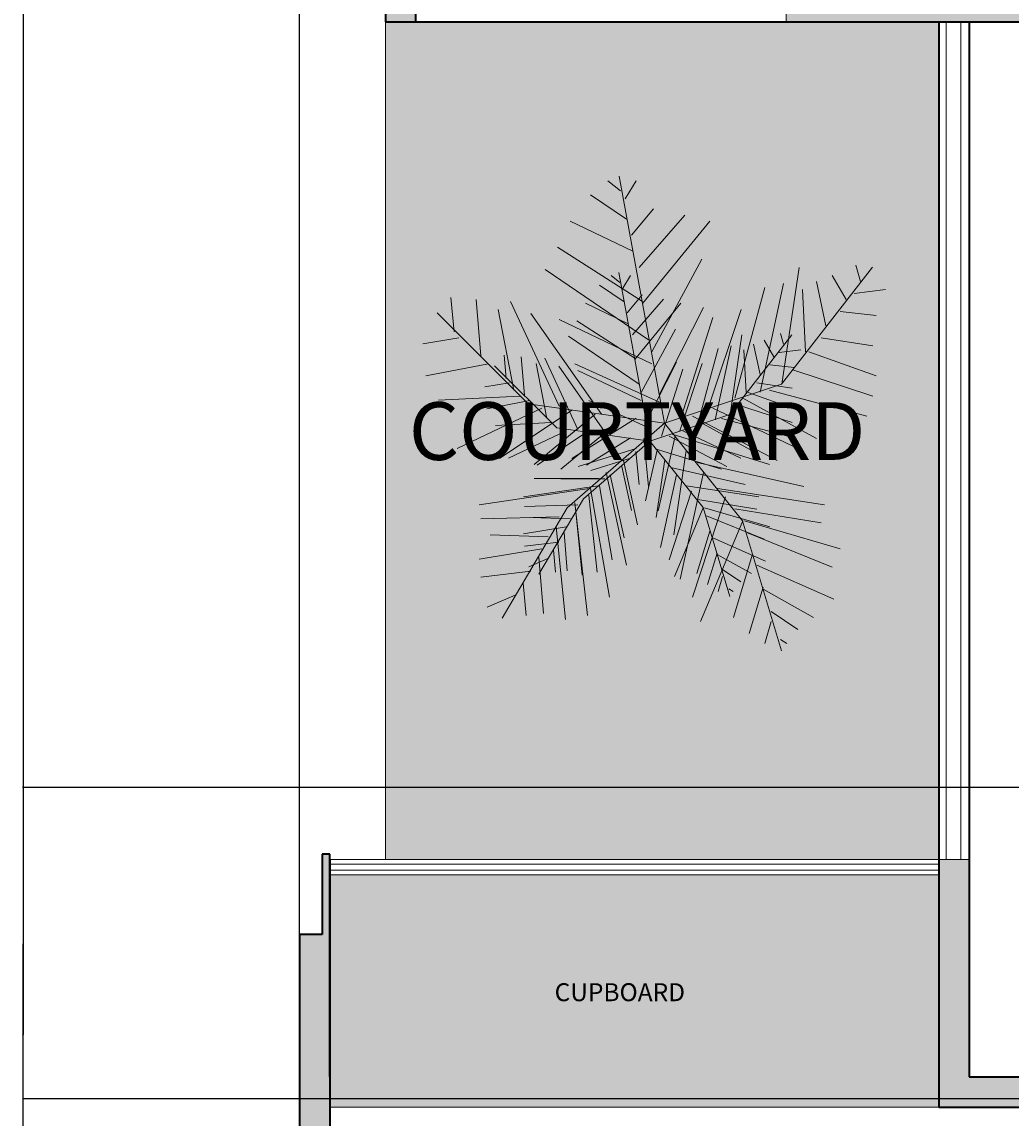
# Model space of a CAD drawing. Units: inches. Extents: x 192 to 1361, y -1362 to 367.
# Tile 14 of 23: x 192 to 487, y -454 to -127. Entities that reach past the tile are written whole.
import ezdxf

# ---------------------------------------------------------------- set-up
doc = ezdxf.new("R2010")
doc.units = ezdxf.units.IN
doc.header["$MEASUREMENT"] = 0
for name, color, linetype, lineweight in [('A-ANNO-DIMS', 2, 'Continuous', 18), ('A-AREA-IDEN', 7, 'Continuous', 18), ('A-WALL-PATT', 250, 'Continuous', 13), ('closet', 32, 'Continuous', 18), ('lawn', 96, 'Continuous', 13), ('text', 7, 'Continuous', 18), ('walls', 7, 'Continuous', 35), ('windows', 4, 'Continuous', 18)]:
    doc.layers.add(name, color=color, linetype=linetype, lineweight=lineweight)
doc.layers.add('A-FLOR-CASE-PATT', color=9, linetype='Continuous', lineweight=13, true_color=0xc7c8ca)
doc.layers.add('L-PLNT-PATT', color=251, linetype='Continuous', lineweight=13, true_color=0x636466)
doc.styles.get("Standard").update_dxf_attribs({"font": 'arial.ttf'})
doc.dimstyles.get("Standard").update_dxf_attribs({"dimtxt": 0.18, "dimasz": 0.18, "dimexe": 0.18, "dimexo": 0.0625, "dimgap": 0.09, "dimtad": 0, "dimtih": 1, "dimtoh": 1, "dimzin": 0, "dimdsep": 46, "dimlunit": 3, "dimtxsty": 'Standard', "dimcen": 0.09, "dimadec": 0, "dimazin": 0, "dimtfac": 1, "dimtofl": 0, "dimtmove": 0, "dimatfit": 3, "dimfxl": 1, "dimtolj": 1, "dimtzin": 0, "dimarcsym": 0})

# ---------------------------------------------------------------- blocks, each defined once
blk = doc.blocks.new('*U4')
for p, q in [((-10.186, 53.64), (-13.084, 55.962)), ((0, 0), (-10.5, 57)), ((-9.099, 51.782), (-6.563, 55.962)), ((-8.737, 47.138), (-17.069, 52.711)), ((-7.65, 43.423), (-2.578, 49.46)), ((-7.288, 39.707), (-21.778, 46.673)), ((-5.839, 35.992), (4.667, 48.067)), ((-5.114, 27.632), (10.463, 46.673)), ((-5.114, 28.097), (-24.676, 40.636)), ((-3.665, 19.273), (-27.574, 35.527)), ((-2.941, 16.486), (8.652, 37.85)), ((27, 9), (48, 36)), ((27.127, 9.056), (31.112, 35.992)), ((44.153, 36.456), (45.239, 32.741)), ((38.719, 34.134), (41.979, 28.561)), ((16.259, 5.805), (23.142, 31.348)), ((22.055, 7.198), (27.489, 32.277)), ((31.836, 30.883), (32.561, 16.486)), ((35.096, 32.741), (37.27, 22.524)), ((43.791, 29.954), (51.036, 30.883)), ((-48.585, 21.131), (-49.309, 29.026)), ((-43.513, 28.561), (-42.427, 15.558)), ((-35.544, 28.097), (-24.314, 3.947)), ((-31.5, 4.5), (-52.5, 25.5)), ((-38.442, 26.239), (-34.819, 7.663)), ((-14.533, 2.09), (-30.834, 25.31)), ((-1.129, 6.734), (9.014, 26.704)), ((10.101, 3.483), (17.708, 26.239)), ((40.53, 25.775), (48.862, 24.846)), ((-24.314, 23.917), (-2.941, 13.7)), ((3.942, 1.625), (11.187, 24.381)), ((-47.498, 19.737), (-55.83, 18.344)), ((36.183, 19.737), (48.137, 17.88)), ((33.285, 16.486), (48.862, 10.913)), ((-40.615, 13.7), (-55.105, 10.913)), ((-20.691, 13.7), (-1.129, 4.876)), ((29.662, 12.307), (48.137, 6.269)), ((0, 0), (27, 9)), ((24.229, 7.663), (46.688, 1.625)), ((-33.37, 6.269), (-52.207, 5.34)), ((18.07, 5.805), (35.096, -3.483)), ((-28.299, 3.483), (-47.86, -5.805)), ((-21.416, 3.018), (-38.079, -8.128)), ((0, 0), (-31.5, 4.5)), ((11.187, 3.483), (30.749, -5.805)), ((-15.982, 2.09), (-30.11, -9.521)), ((0, 0), (-22.5, -19.5)), ((-6.563, 1.161), (-21.416, -8.128)), ((0, 0), (18, -22.5)), ((6.478, 1.625), (26.04, -8.592)), ((-4.752, -3.483), (-3.665, -14.629)), ((2.493, -3.019), (-1.491, -20.202)), ((1.769, -2.555), (24.229, -9.521)), ((-6.563, -5.805), (-19.967, -9.985)), ((5.029, -6.27), (2.131, -25.775)), ((-9.461, -8.592), (-6.201, -23.453)), ((7.565, -9.056), (32.198, -14.629)), ((-13.446, -11.378), (-8.737, -32.741)), ((9.014, -11.378), (3.58, -35.992)), ((-17.431, -15.094), (-42.789, -18.809)), ((-15.257, -12.772), (-30.11, -12.772)), ((-17.069, -15.094), (-12.721, -40.172)), ((12.274, -15.094), (36.907, -18.809)), ((14.085, -16.951), (6.478, -40.172)), ((-22.5, -19.5), (-37.5, -45)), ((-20.691, -18.345), (-17.793, -44.352)), ((16.259, -19.738), (36.183, -22.989)), ((-24.314, -21.596), (-42.427, -22.06)), ((18.07, -22.524), (8.289, -45.745)), ((18, -22.5), (27, -52.5)), ((18.433, -22.524), (40.53, -29.026)), ((-25.038, -23.918), (-22.865, -45.281)), ((-26.849, -26.24), (-40.253, -25.775)), ((19.157, -25.311), (38.719, -33.206)), ((-28.299, -29.026), (-42.789, -31.348)), ((-29.023, -30.884), (-27.936, -43.887)), ((20.244, -30.419), (15.897, -44.816)), ((21.331, -32.741), (39.081, -40.636)), ((-30.834, -34.135), (-42.427, -35.528)), ((-32.646, -36.921), (-31.921, -44.352)), ((22.78, -37.85), (19.519, -48.532)), ((-34.457, -39.708), (-40.978, -42.494)), ((22.78, -38.314), (34.372, -44.816)), ((24.591, -43.423), (30.749, -47.603)), ((24.591, -45.745), (23.142, -50.854)), ((26.764, -49.925), (28.213, -50.854))]:
    blk.add_line(p, q)
blk = doc.blocks.new('*D48')
at = {"layer": 'A-ANNO-DIMS', "color": 0, "lineweight": -2, "transparency": 16777216}
for p, q in [((325.63, 258.53), (192.16, 258.53)), ((192.34, 258.35), (192.34, -429.22)), ((192.34, -1117.14), (192.34, -429.58)), ((395.21, -1117.32), (192.16, -1117.32))]:
    blk.add_line(p, q, dxfattribs=at)
at = {"layer": 'A-ANNO-DIMS', "color": 0, "transparency": 16777216}
for points in [[(192.31, 258.35), (192.37, 258.35), (192.34, 258.53)], [(192.31, -1117.14), (192.37, -1117.14), (192.34, -1117.32)]]:
    blk.add_solid(points, dxfattribs=at)
at = {"layer": 'Defpoints', "color": 0, "transparency": 16777216}
for p in [(325.7, 258.53), (192.34, -1117.32), (395.28, -1117.32)]:
    blk.add_point(p, dxfattribs=at)
at = {"layer": 'A-ANNO-DIMS', "color": 0, "transparency": 16777216, "insert": (192.34, -429.4), "char_height": 0.18, "attachment_point": 5}
blk.add_mtext('\\A1;1375.9', dxfattribs=at)
blk = doc.blocks.new('*D49')
at = {"layer": 'A-ANNO-DIMS', "color": 0, "lineweight": -2, "transparency": 16777216}
for p, q in [((274.89, -399.35), (274.89, 367.39)), ((275.07, 367.21), (287.25, 367.21)), ((300.37, 367.21), (288.18, 367.21)), ((300.55, 191.16), (300.55, 367.39))]:
    blk.add_line(p, q, dxfattribs=at)
at = {"layer": 'A-ANNO-DIMS', "color": 0, "transparency": 16777216}
for points in [[(275.07, 367.24), (275.07, 367.18), (274.89, 367.21)], [(300.37, 367.24), (300.37, 367.18), (300.55, 367.21)]]:
    blk.add_solid(points, dxfattribs=at)
at = {"layer": 'Defpoints', "color": 0, "transparency": 16777216}
for p in [(300.55, 367.21), (300.55, 191.1), (274.89, -399.41)]:
    blk.add_point(p, dxfattribs=at)
at = {"layer": 'A-ANNO-DIMS', "color": 0, "transparency": 16777216, "insert": (287.72, 367.21), "char_height": 0.18, "attachment_point": 5}
blk.add_mtext('\\A1;25.653', dxfattribs=at)
blk = doc.blocks.new('*D71')
at = {"layer": 'A-ANNO-DIMS', "color": 0, "lineweight": -2, "transparency": 16777216}
for p, q in [((784.74, -355.5), (192.16, -355.5)), ((192.34, -355.68), (192.34, -401.82)), ((192.34, -448.32), (192.34, -402.18)), ((784.74, -448.5), (192.16, -448.5))]:
    blk.add_line(p, q, dxfattribs=at)
at = {"layer": 'A-ANNO-DIMS', "color": 0, "transparency": 16777216}
for points in [[(192.31, -355.68), (192.37, -355.68), (192.34, -355.5)], [(192.31, -448.32), (192.37, -448.32), (192.34, -448.5)]]:
    blk.add_solid(points, dxfattribs=at)
at = {"layer": 'Defpoints', "color": 0, "transparency": 16777216}
for p in [(784.8, -355.5), (192.34, -448.5), (784.8, -448.5)]:
    blk.add_point(p, dxfattribs=at)
at = {"layer": 'A-ANNO-DIMS', "color": 0, "transparency": 16777216, "insert": (192.34, -402), "char_height": 0.18, "attachment_point": 5}
blk.add_mtext('\\A1;93', dxfattribs=at)

msp = doc.modelspace()

# ---------------------------------------------------------------- hatches: boundary and pattern name
at = {"layer": 'A-FLOR-CASE-PATT'}
h = msp.add_hatch(color=256, dxfattribs=at)
h.dxf.hatch_style = 1
h.paths.add_polyline_path([(465.8041, -381.5384), (283.8925, -381.5384), (283.8925, -441.898), (283.8925, -450.898), (465.8041, -450.898)])
at = {"layer": 'A-WALL-PATT'}
h = msp.add_hatch(color=256, dxfattribs=at)
h.dxf.hatch_style = 1
h.paths.add_polyline_path([(309.5452, 191.102), (300.5452, 191.102), (300.5452, -126.898), (309.5452, -126.898), (309.5452, -117.898)])
h.paths.add_polyline_path([(420.798, 191.102), (337.3229, 191.102), (337.3229, 182.102), (420.798, 182.102)])
h.paths.add_polyline_path([(518.5452, 182.102), (625.4022, 182.102), (625.4022, 191.102), (509.5452, 191.102), (509.5452, 114.3262), (518.5452, 114.3262)])
h.paths.add_polyline_path([(842.5452, 191.102), (763.4438, 191.102), (763.4438, 182.102), (833.5452, 182.102), (833.5452, 161.1615), (836.8088, 161.1615), (842.5452, 161.1615)])
h.paths.add_polyline_path([(842.5452, -16.5675), (833.5452, -16.5675), (833.5452, -60.4996), (784.8041, -60.4996), (784.8041, -354.6796), (793.8041, -354.6796), (793.8041, -69.4996), (1094.1252, -69.4996), (1094.1252, -60.4996), (842.5452, -60.4996)])
h.paths.add_polyline_path([(518.5452, 36.602), (509.5452, 36.602), (509.5452, -117.898), (420.2204, -117.898), (420.2204, -126.898), (518.5452, -126.898)])
h.paths.add_polyline_path([(474.8041, -377.0384), (465.8041, -377.0384), (465.8041, -381.5384), (465.8041, -450.898), (537.5717, -450.898), (537.5717, -441.898), (474.8041, -441.898)])
h.paths.add_polyline_path([(1162.8041, -380.6763), (1204.3001, -380.6763), (1204.3001, -375.6763), (1195.1471, -375.6763), (1153.8041, -375.6763), (1153.8041, -448.4996), (856.5691, -448.4996), (856.5691, -457.4996), (1162.8041, -457.4996)])
h.paths.add_polyline_path([(1162.8041, -525.128), (1153.8041, -525.128), (1153.8041, -597.4996), (1162.8041, -597.4996)], flags=17)
h.paths.add_polyline_path([(1162.8041, -60.4996), (1153.8041, -60.4996), (1153.8041, -69.4996), (1153.8041, -177.4733), (1205.8889, -177.4733), (1205.8889, -172.4733), (1162.8041, -172.4733)])
h.paths.add_polyline_path([(980.5799, -525.686), (971.5799, -525.686), (971.5799, -597.4996), (980.5799, -597.4996)], flags=17)
h.paths.add_polyline_path([(856.5691, -448.4996), (798.7542, -448.4996), (784.8041, -448.4996), (784.8041, -457.4996), (847.5691, -457.4996), (847.5691, -597.4996), (784.8041, -597.4996), (784.8041, -606.4996), (1273.5658, -606.4996), (1273.5658, -597.4996), (856.5691, -597.4996)])
h.paths.add_polyline_path([(1273.5658, -773.892), (1099.8366, -773.892), (1099.8366, -851.9362), (1108.8366, -851.9362), (1108.8366, -782.892), (1273.5658, -782.892)])
h.paths.add_polyline_path([(1108.8366, -982.9214), (1099.8366, -982.9214), (1099.8366, -1067.6246), (1037.7563, -1067.6246), (1037.7563, -1076.6246), (1108.8366, -1076.6246)])
h.paths.add_polyline_path([(835.078, -1067.6246), (758.8458, -1067.6246), (758.8458, -940.2324), (749.8458, -940.2324), (749.8458, -963.172), (749.8458, -970.4644), (749.8458, -1076.6246), (835.078, -1076.6246)])
h.paths.add_polyline_path([(450.307, -1066.9838), (441.307, -1066.9838), (441.307, -1076.6246), (450.307, -1076.6246)])
h.paths.add_polyline_path([(492.8925, -756.4415), (274.8925, -756.4415), (274.8925, -765.4415), (492.8925, -765.4415)])
h.paths.add_polyline_path([(283.8925, -835.2244), (274.8925, -835.2244), (274.8925, -914.4415), (492.8925, -914.4415), (492.8925, -839.9415), (483.8925, -839.9415), (483.8925, -905.4415), (283.8925, -905.4415)])
h.paths.add_polyline_path([(283.8925, -441.898), (283.8925, -375.4296), (281.6021, -375.4296), (281.6021, -399.4121), (274.8925, -399.4121), (274.8925, -441.898), (274.8925, -684.5089), (283.8925, -684.5089)])
at = {"layer": 'L-PLNT-PATT'}
h = msp.add_hatch(color=256, dxfattribs=at)
h.dxf.hatch_style = 1
h.paths.add_polyline_path([(465.8041, -126.898), (300.5452, -126.898), (300.5452, -377.0384), (465.8041, -377.0384)])

# ---------------------------------------------------------------- linework, layer by layer
at = {"layer": 'closet'}
msp.add_line((465.8041, -450.898), (283.8925, -450.898), dxfattribs=at)
at = {"layer": 'lawn'}
msp.add_line((300.5452, -126.898), (300.5452, -377.0384), dxfattribs=at)
at = {"layer": 'walls'}
for p, q in [((300.5452, 191.102), (300.5452, -126.898)), ((309.5452, 191.102), (309.5452, -126.898)), ((300.5452, -126.898), (518.5452, -126.898)), ((465.8041, -126.898), (465.8041, -450.898)), ((474.8041, -126.898), (474.8041, -441.898)), ((283.8925, -375.4296), (281.6021, -375.4296)), ((281.6021, -375.4296), (281.6021, -399.4121)), ((283.8925, -441.898), (283.8925, -375.4296)), ((283.8925, -377.0384), (283.8925, -441.898)), ((281.6021, -399.4121), (274.8925, -399.4121)), ((274.8925, -399.4121), (274.8925, -441.898)), ((274.8925, -441.898), (274.8925, -914.4415)), ((283.8925, -441.898), (283.8925, -756.4415)), ((474.8041, -441.898), (537.5717, -441.898)), ((465.8041, -450.898), (537.5717, -450.898))]:
    msp.add_line(p, q, dxfattribs=at)
at = {"layer": 'windows'}
for p, q in [((309.5452, -117.898), (309.5452, -126.898)), ((420.2204, -117.898), (420.2204, -126.898)), ((474.8041, -126.898), (465.8041, -126.898)), ((467.9611, -377.0384), (467.9611, -126.898)), ((472.3709, -377.0384), (472.3709, -126.898)), ((472.3709, -126.898), (474.8041, -126.898)), ((300.5452, -377.0384), (283.8925, -377.0384)), ((283.8925, -377.0384), (283.8925, -381.5384)), ((283.8925, -381.5384), (283.8925, -378.4233)), ((283.8925, -378.4233), (465.8041, -378.4233)), ((465.8041, -377.0384), (300.5452, -377.0384)), ((465.8041, -378.4233), (465.8041, -377.0384)), ((465.8041, -377.0384), (465.8041, -381.5384)), ((465.8041, -377.0384), (474.8041, -377.0384)), ((465.8041, -380.1648), (283.8925, -380.1648)), ((465.8041, -381.5384), (283.8925, -381.5384)), ((465.8041, -381.5384), (465.8041, -380.1648))]:
    msp.add_line(p, q, dxfattribs=at)

# ---------------------------------------------------------------- block references
at = {"layer": 'lawn'}
for p, xscale, yscale, zscale in [((383.8639, -246.729), 1.293445435691037, 1.293445435691037, 1.293445435691037), ((379.4904, -252.0686), 0.8828807890770264, 0.8828807890770264, 0.8828807890770264)]:
    msp.add_blockref('*U4', p, dxfattribs=dict(at, xscale=xscale, yscale=yscale, zscale=zscale))

# ---------------------------------------------------------------- texts
at = {"layer": 'A-AREA-IDEN'}
msp.add_text('COURTYARD', height=17.23824, dxfattribs=at).set_placement((307.5238, -257.691))
at = {"layer": 'text'}
msp.add_text('CUPBOARD', height=5.36502, dxfattribs=at).set_placement((351.0459, -419.3009))

# ---------------------------------------------------------------- dimensions: what is measured, and where the dimension line sits
at = {"layer": 'A-ANNO-DIMS'}
dim = msp.add_linear_dim(base=(300.5452, 367.2097), p1=(274.8925, -399.4121), p2=(300.5452, 191.102), dimstyle='Standard', override={"dimdec": 3, "dimlfac": 1, "dimrnd": 0, "dimzin": 0, "dimdsep": 46, "dimlunit": 2}, dxfattribs=at)
dim.commit()
dim.dimension.update_dxf_attribs({"geometry": '*D49', "text_midpoint": (287.7189, 367.2097)})
for base, p1, p2, override, picture, middle in [((192.3425, -1117.3227), (325.6957, 258.5286), (395.2768, -1117.3227), {"dimdec": 1, "dimlfac": 1, "dimrnd": 0, "dimzin": 0, "dimdsep": 46, "dimlunit": 2}, '*D48', (192.3425, -429.3971)), ((192.3425, -448.4996), (784.8041, -355.4994), (784.8041, -448.4996), {"dimdec": 0, "dimlfac": 1, "dimrnd": 0, "dimzin": 0, "dimdsep": 46, "dimlunit": 2}, '*D71', (192.3425, -401.9995))]:
    dim = msp.add_linear_dim(base=base, p1=p1, p2=p2, angle=90, dimstyle='Standard', override=override, dxfattribs=at)
    dim.commit()
    dim.dimension.update_dxf_attribs({"geometry": picture, "text_midpoint": middle})

doc.saveas('drawing.dxf')
